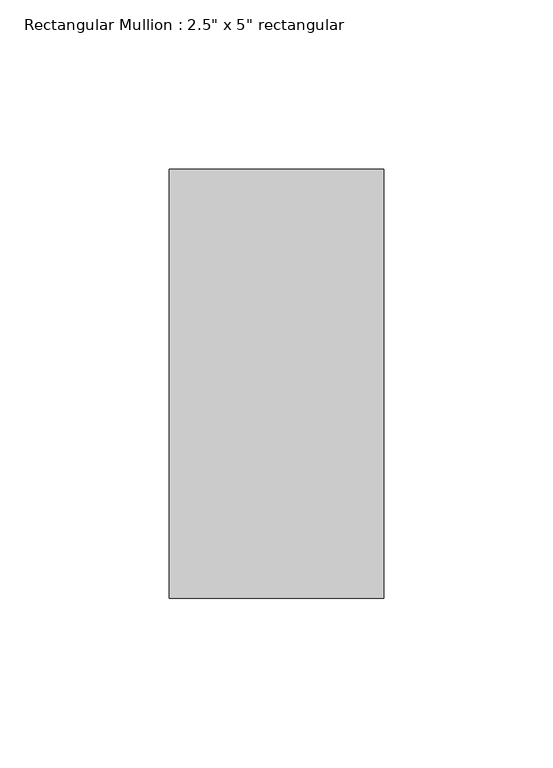
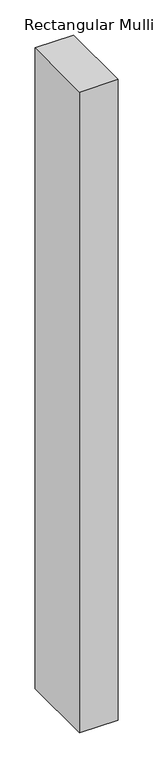
"""IFC4 building model written with IfcOpenShell, lengths in millimetres: member geometry."""

from ifc_helpers import new_model, si_unit, frame, origin, place, context, project, spatial, polyline, outline, extrude, source, transform, mapped, element, save


def member_05798353(model_context):
    return source(origin(), model_context, "Body", "SweptSolid", [
        extrude(outline(polyline([(0.0, 63.5), (0.0, -63.5), (-63.5, -63.5), (-63.5, 63.5), (0.0, 63.5)])), frame((0.0, 0.0, -1116.5), z_axis=(0.0, 0.0, 1.0), x_axis=(1.0, 0.0, 0.0)), (0.0, 0.0, 1.0), 1116.5),
    ])


if __name__ == "__main__":
    model = new_model("IFC4")
    model_context = context("Model", 3, world=origin())
    ifc_project = project(units=[si_unit("LENGTHUNIT", "METRE", prefix="MILLI")], contexts=[model_context])
    site = spatial("IfcSite", under=ifc_project)
    building = spatial("IfcBuilding", under=site)
    placement = place(None, origin())
    member_shape = member_05798353(model_context)
    element("IfcMember", 1, ObjectType="Rectangular Mullion : 2.5\" x 5\" rectangular", at=placement, inside=building, context=model_context, shape_type="MappedRepresentation", body=[
        mapped(member_shape, transform((0.0, 0.0, 0.0), x_axis=(1.0, 0.0, 0.0), y_axis=(0.0, 1.0, 0.0), z_axis=(0.0, 0.0, 1.0))),
    ])
    save(model, "model.ifc")

# Revit data of these elements
# Type "Rectangular Mullion : 2.5\" x 5\" rectangular"
#   built-in parameter 1007304 = 0.416667 (stored number, unit not read)
#   built-in parameter 1007301 = 0.104167 (stored number, unit not read)
#   built-in parameter 1007300 = 0.104167 (stored number, unit not read)
# Element 1 (IfcMember, "Rectangular Mullion : 2.5\" x 5\" rectangular")
#   Materials on its faces: "Damp-proofing"
# Materials
#   "Damp-proofing": class "Generic", colour RGB 127 127 127, transparency 0, Description = "Damp-proofing", Cost = 0
